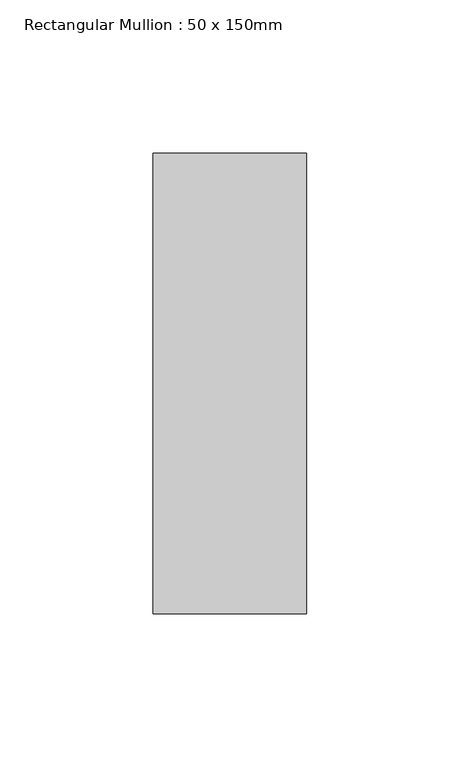
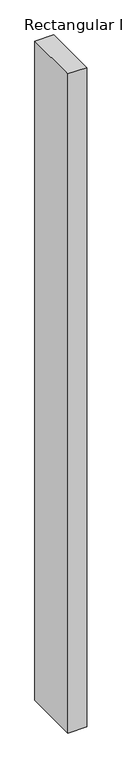
"""IFC4 building model written with IfcOpenShell, lengths in millimetres: member geometry, Rectangular Mullion : 50 x 150mm."""

from ifc_helpers import new_model, si_unit, frame, origin, place, context, project, spatial, polyline, outline, extrude, source, transform, mapped, element, save


def rectangular_mullion_50_x_150mm_c76b6149(model_context):
    return source(origin(), model_context, "Body", "SweptSolid", [
        extrude(outline(polyline([(0.0, 75.0), (0.0, -75.0), (-50.0, -75.0), (-50.0, 75.0), (0.0, 75.0)])), frame((0.0, 0.0, -1828.8), z_axis=(0.0, 0.0, 1.0), x_axis=(1.0, 0.0, 0.0)), (0.0, 0.0, 1.0), 1828.8),
    ])


if __name__ == "__main__":
    model = new_model("IFC4")
    model_context = context("Model", 3, world=origin())
    ifc_project = project(units=[si_unit("LENGTHUNIT", "METRE", prefix="MILLI")], contexts=[model_context])
    site = spatial("IfcSite", under=ifc_project)
    building = spatial("IfcBuilding", under=site)
    placement = place(None, origin())
    rectangular_mullion_50_x_150mm_shape = rectangular_mullion_50_x_150mm_c76b6149(model_context)
    element("IfcMember", 1, ObjectType="Rectangular Mullion : 50 x 150mm", at=placement, inside=building, context=model_context, shape_type="MappedRepresentation", body=[
        mapped(rectangular_mullion_50_x_150mm_shape, transform((0.0, 0.0, 0.0), x_axis=(1.0, 0.0, 0.0), y_axis=(0.0, 1.0, 0.0), z_axis=(0.0, 0.0, 1.0))),
    ])
    save(model, "model.ifc")

# Revit data of these elements
# Type "Rectangular Mullion : 50 x 150mm"
#   built-in parameter 1007304 = 0.492126 (stored number, unit not read)
#   built-in parameter 1007301 = 0.082021 (stored number, unit not read)
#   built-in parameter 1007300 = 0.082021 (stored number, unit not read)
# Element 1 (IfcMember, "Rectangular Mullion : 50 x 150mm")
#   Materials on its faces: "Aluminium"
# Materials
#   "Aluminium": class "Metal", colour RGB 247 247 247, transparency 0, Description = "Aluminium 6061", Cost = 0
